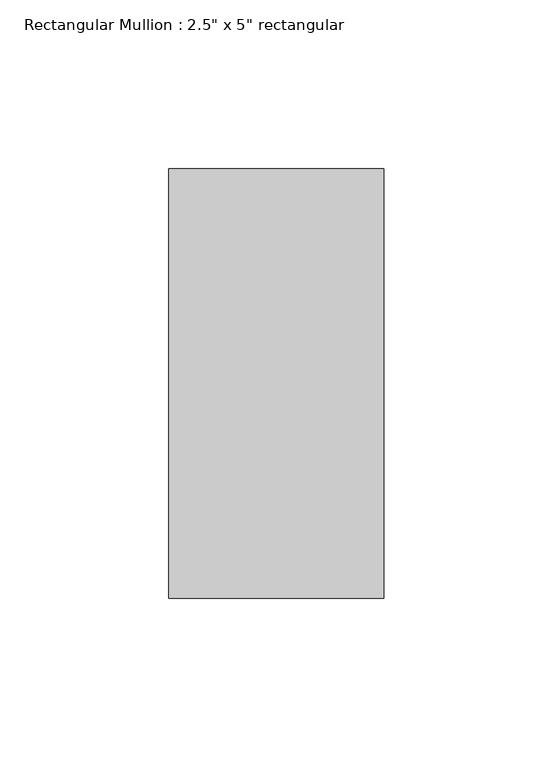
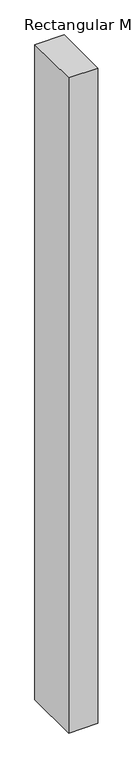
"""IFC4 building model written with IfcOpenShell, lengths in millimetres: member geometry."""

from ifc_helpers import new_model, si_unit, frame, origin, place, context, project, spatial, polyline, outline, extrude, source, transform, mapped, element, save


def member_2ab56126(model_context):
    return source(origin(), model_context, "Body", "SweptSolid", [
        extrude(outline(polyline([(31.75, 63.5), (31.75, -63.5), (-31.75, -63.5), (-31.75, 63.5), (31.75, 63.5)])), frame((0.0, 0.0, -1510.5980535), z_axis=(0.0, 0.0, 1.0), x_axis=(1.0, 0.0, 0.0)), (0.0, 0.0, 1.0), 1510.5980535),
    ])


if __name__ == "__main__":
    model = new_model("IFC4")
    model_context = context("Model", 3, world=origin())
    ifc_project = project(units=[si_unit("LENGTHUNIT", "METRE", prefix="MILLI")], contexts=[model_context])
    site = spatial("IfcSite", under=ifc_project)
    building = spatial("IfcBuilding", under=site)
    placement = place(None, origin())
    member_shape = member_2ab56126(model_context)
    element("IfcMember", 1, ObjectType="Rectangular Mullion : 2.5\" x 5\" rectangular", at=placement, inside=building, context=model_context, shape_type="MappedRepresentation", body=[
        mapped(member_shape, transform((0.0, 0.0, 0.0), x_axis=(1.0, 0.0, 0.0), y_axis=(0.0, 1.0, 0.0), z_axis=(0.0, 0.0, 1.0))),
    ])
    save(model, "model.ifc")

# Revit data of these elements
# Type "Rectangular Mullion : 2.5\" x 5\" rectangular"
#   built-in parameter 1007304 = 0.416667 (stored number, unit not read)
#   built-in parameter 1007301 = 0.104167 (stored number, unit not read)
#   built-in parameter 1007300 = 0.104167 (stored number, unit not read)
# Element 1 (IfcMember, "Rectangular Mullion : 2.5\" x 5\" rectangular")
#   Materials on its faces: "Aluminum"
# Materials
#   "Aluminum": class "Metal", colour RGB 247 247 247, transparency 0, Description = "Aluminum 6061", Cost = 0
